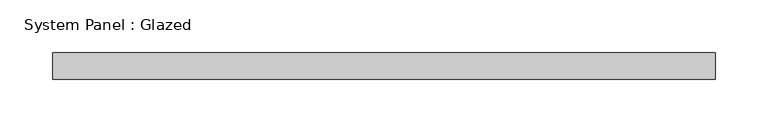
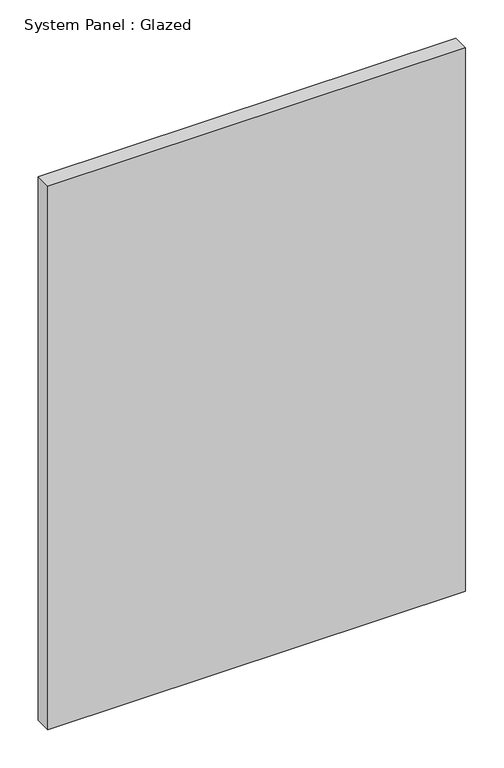
"""IFC4 building model written with IfcOpenShell, lengths in millimetres: plate geometry, System Panel : Glazed."""

from ifc_helpers import new_model, si_unit, origin, origin_with_axes, place, context, project, spatial, polyline, outline, extrude, source, transform, mapped, element, save


def system_panel_glazed_36803b61(model_context):
    return source(origin(), model_context, "Body", "SweptSolid", [
        extrude(outline(polyline([(314.325, 24.5), (-314.325, 24.5), (-314.325, 49.5), (314.325, 49.5), (314.325, 24.5)])), origin_with_axes(), (0.0, 0.0, 1.0), 864.4),
    ])


if __name__ == "__main__":
    model = new_model("IFC4")
    model_context = context("Model", 3, world=origin())
    ifc_project = project(units=[si_unit("LENGTHUNIT", "METRE", prefix="MILLI")], contexts=[model_context])
    site = spatial("IfcSite", under=ifc_project)
    building = spatial("IfcBuilding", under=site)
    placement = place(None, origin())
    system_panel_glazed_shape = system_panel_glazed_36803b61(model_context)
    element("IfcPlate", 1, ObjectType="System Panel : Glazed", at=placement, inside=building, context=model_context, shape_type="MappedRepresentation", body=[
        mapped(system_panel_glazed_shape, transform((0.0, 0.0, 0.0), x_axis=(1.0, 0.0, 0.0), y_axis=(0.0, 1.0, 0.0), z_axis=(0.0, 0.0, 1.0))),
    ])
    save(model, "model.ifc")

# Revit data of these elements
# Type "System Panel : Glazed"
#   Keynote = "H11"
#   Construction Type Id = "GSP4R"
#   Analytic Construction = "1/8 in Pilkington single glazing"
#   Visual Light Transmittance = 0.9
#   Solar Heat Gain Coefficient = 0.86
#   Heat Transfer Coefficient (U) = 6.7069 W/(m²·K)
#   Define Thermal Properties by = 1
# Element 1 (IfcPlate, "System Panel : Glazed")
#   Materials on its faces: "Glass"
# Materials
#   "Glass": class "Glass", colour RGB 0 128 192, transparency 0.9, Description = "Soda Lime Glass", Cost = 0
